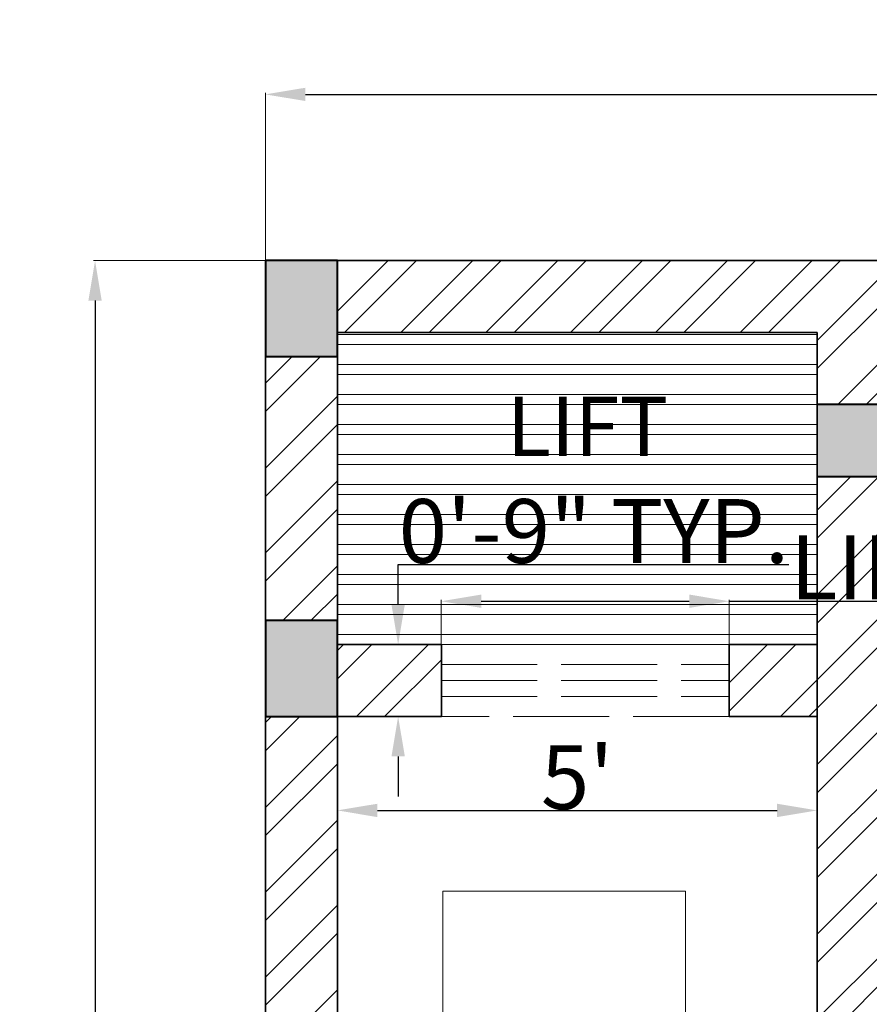
# Model space of a CAD drawing. Units: inches. Extents: x 351 to 1738, y -265 to 286.
# Tile 26 of 38: x 1004 to 1110, y 163 to 286. Entities that reach past the tile are written whole.
import ezdxf

# ---------------------------------------------------------------- set-up
doc = ezdxf.new("R2010")
doc.units = ezdxf.units.IN
doc.header["$MEASUREMENT"] = 0
doc.linetypes.add('ACAD_ISO02W100', pattern=[15, 12, -3])
for name, color, linetype, lineweight in [('A-ANNO-DIMS', 2, 'Continuous', 18), ('A-ANNO-SYMB', 7, 'Continuous', 18), ('A-AREA-IDEN', 7, 'Continuous', 18), ('A-COLS', 7, 'Continuous', 40), ('A-COLS-PATT', 6, 'Continuous', 13), ('A-FLOR-EVTR', 242, 'ACAD_ISO02W100', 18), ('A-FLOR-EVTR-PATT', 9, 'Continuous', 9), ('A-WALL', 7, 'Continuous', 35), ('A-WALL-PATT', 152, 'Continuous', 13)]:
    doc.layers.add(name, color=color, linetype=linetype, lineweight=lineweight)
doc.styles.add('Annotative', font='arial.ttf')
doc.styles.get("Standard").update_dxf_attribs({"font": 'arial.ttf'})
doc.dimstyles.get("Standard").update_dxf_attribs({"dimtxt": 8, "dimasz": 5, "dimexe": 0.18, "dimexo": 0.0625, "dimgap": 0.09, "dimtad": 1, "dimtoh": 1, "dimzin": 0, "dimdsep": 46, "dimlunit": 4, "dimtxsty": 'Standard', "dimcen": 0, "dimclre": 256, "dimadec": 0, "dimazin": 0, "dimtfac": 1, "dimtofl": 0, "dimtmove": 0, "dimatfit": 3, "dimfxl": 1, "dimtolj": 1, "dimtzin": 0, "dimlwe": -1, "dimarcsym": 0})

# ---------------------------------------------------------------- blocks, each defined once
blk = doc.blocks.new('*D7')
at = {"layer": 'A-ANNO-DIMS', "color": 0, "transparency": 16777216}
for p, q in [((1034.7, 256.03), (1034.7, 276.92)), ((1566.7, 256.03), (1566.7, 276.92))]:
    blk.add_line(p, q, dxfattribs=at)
at = {"layer": 'A-ANNO-DIMS', "color": 0, "lineweight": -2, "transparency": 16777216}
blk.add_line((1039.7, 276.74), (1561.7, 276.74), dxfattribs=at)
at = {"layer": 'A-ANNO-DIMS', "color": 0, "transparency": 16777216}
for points in [[(1039.7, 277.57), (1039.7, 275.91), (1034.7, 276.74)], [(1561.7, 277.57), (1561.7, 275.91), (1566.7, 276.74)]]:
    blk.add_solid(points, dxfattribs=at)
at = {"layer": 'Defpoints', "color": 0, "transparency": 16777216}
for p in [(1566.7, 276.74), (1034.7, 255.96), (1566.7, 255.96)]:
    blk.add_point(p, dxfattribs=at)
at = {"layer": 'A-ANNO-DIMS', "color": 0, "transparency": 16777216, "insert": (1300.7, 280.83), "char_height": 8, "attachment_point": 5}
blk.add_mtext('\\A1;44\'-4"', dxfattribs=at)
blk = doc.blocks.new('*D8')
at = {"layer": 'A-ANNO-DIMS', "color": 0, "transparency": 16777216}
for p, q in [((1034.64, 255.96), (1013.22, 255.96)), ((1034.64, -203.04), (1013.22, -203.04))]:
    blk.add_line(p, q, dxfattribs=at)
at = {"layer": 'A-ANNO-DIMS', "color": 0, "lineweight": -2, "transparency": 16777216}
blk.add_line((1013.4, 250.96), (1013.4, -198.04), dxfattribs=at)
at = {"layer": 'A-ANNO-DIMS', "color": 0, "transparency": 16777216}
for points in [[(1012.57, 250.96), (1014.23, 250.96), (1013.4, 255.96)], [(1012.57, -198.04), (1014.23, -198.04), (1013.4, -203.04)]]:
    blk.add_solid(points, dxfattribs=at)
at = {"layer": 'Defpoints', "color": 0, "transparency": 16777216}
for p in [(1034.7, 255.96), (1013.4, -203.04), (1034.7, -203.04)]:
    blk.add_point(p, dxfattribs=at)
at = {"layer": 'A-ANNO-DIMS', "color": 0, "transparency": 16777216, "insert": (1009.22, 26.46), "char_height": 8, "attachment_point": 5, "rotation": 90}
blk.add_mtext('\\A1;38\'-3"', dxfattribs=at)
blk = doc.blocks.new('*D11')
at = {"layer": 'A-ANNO-DIMS', "color": 0, "transparency": 16777216}
for p, q in [((1043.7, 198.9), (1043.7, 187.03)), ((1103.7, 198.9), (1103.7, 187.03))]:
    blk.add_line(p, q, dxfattribs=at)
at = {"layer": 'A-ANNO-DIMS', "color": 0, "lineweight": -2, "transparency": 16777216}
blk.add_line((1048.7, 187.21), (1098.7, 187.21), dxfattribs=at)
at = {"layer": 'A-ANNO-DIMS', "color": 0, "transparency": 16777216}
for points in [[(1048.7, 188.04), (1048.7, 186.37), (1043.7, 187.21)], [(1098.7, 188.04), (1098.7, 186.37), (1103.7, 187.21)]]:
    blk.add_solid(points, dxfattribs=at)
at = {"layer": 'Defpoints', "color": 0, "transparency": 16777216}
for p in [(1043.7, 198.96), (1103.7, 198.96), (1103.7, 187.21)]:
    blk.add_point(p, dxfattribs=at)
at = {"layer": 'A-ANNO-DIMS', "color": 0, "transparency": 16777216, "insert": (1073.7, 191.36), "char_height": 8, "attachment_point": 5}
blk.add_mtext("\\A1;5'", dxfattribs=at)
blk = doc.blocks.new('COL-9x12')
blk.add_lwpolyline([(0, 12), (0, 0), (9, 0), (9, 12)], close=True)
blk = doc.blocks.new('LIFT-DOOR-36')
for p, q in [((0, 9), (36, 9)), ((0, 6.5), (36, 6.5)), ((0, 4.5), (36, 4.5)), ((0, 2.5), (36, 2.5)), ((36, 0), (0, 0))]:
    blk.add_line(p, q)
blk = doc.blocks.new('*D54')
at = {"layer": 'A-ANNO-DIMS', "transparency": 16777216}
for p, q in [((1056.7, 208.03), (1056.7, 213.54)), ((1092.7, 208.03), (1092.7, 213.54))]:
    blk.add_line(p, q, dxfattribs=at)
at = {"layer": 'A-ANNO-DIMS', "color": 0, "lineweight": -2, "transparency": 16777216}
for p, q in [((1061.7, 213.36), (1087.7, 213.36)), ((1092.7, 213.36), (1209.01, 213.36))]:
    blk.add_line(p, q, dxfattribs=at)
at = {"layer": 'A-ANNO-DIMS', "color": 0, "transparency": 16777216}
for points in [[(1061.7, 214.2), (1061.7, 212.53), (1056.7, 213.36)], [(1087.7, 214.2), (1087.7, 212.53), (1092.7, 213.36)]]:
    blk.add_solid(points, dxfattribs=at)
at = {"layer": 'Defpoints', "color": 0, "transparency": 16777216}
for p in [(1092.7, 213.36), (1056.7, 207.96), (1092.7, 207.96)]:
    blk.add_point(p, dxfattribs=at)
at = {"layer": 'A-ANNO-DIMS', "color": 0, "transparency": 16777216, "insert": (1153.35, 217.59), "char_height": 8, "attachment_point": 5}
blk.add_mtext('\\A1;LIFT DOOR 3\'-0" TYP.', dxfattribs=at)
blk = doc.blocks.new('*D55')
at = {"layer": 'A-ANNO-DIMS', "color": 0, "lineweight": -2, "transparency": 16777216}
for p, q in [((1051.3, 212.96), (1051.3, 217.96)), ((1051.3, 217.96), (1100.16, 217.96)), ((1051.3, 193.96), (1051.3, 188.96))]:
    blk.add_line(p, q, dxfattribs=at)
at = {"layer": 'A-ANNO-DIMS', "transparency": 16777216}
for p, q in [((1056.64, 207.96), (1051.12, 207.96)), ((1056.64, 198.96), (1051.12, 198.96))]:
    blk.add_line(p, q, dxfattribs=at)
at = {"layer": 'A-ANNO-DIMS', "color": 0, "transparency": 16777216}
for points in [[(1050.47, 212.96), (1052.14, 212.96), (1051.3, 207.96)], [(1050.47, 193.96), (1052.14, 193.96), (1051.3, 198.96)]]:
    blk.add_solid(points, dxfattribs=at)
at = {"layer": 'Defpoints', "color": 0, "transparency": 16777216}
for p in [(1051.3, 207.96), (1056.7, 207.96), (1056.7, 198.96)]:
    blk.add_point(p, dxfattribs=at)
at = {"layer": 'A-ANNO-DIMS', "color": 0, "transparency": 16777216, "insert": (1075.78, 222.14), "char_height": 8, "attachment_point": 5}
blk.add_mtext('\\A1;0\'-9" TYP.', dxfattribs=at)

msp = doc.modelspace()

# ---------------------------------------------------------------- hatches: boundary and pattern name
at = {"layer": 'A-COLS-PATT'}
h = msp.add_hatch(color=256, dxfattribs=at)
h.dxf.hatch_style = 1
h.paths.add_polyline_path([(1112.704, 237.963), (1103.704, 237.963), (1103.704, 228.963), (1112.704, 228.963)])
h.paths.add_polyline_path([(1115.704, 237.963), (1112.704, 237.963), (1112.704, 228.963), (1115.704, 228.963)])
h.paths.add_polyline_path([(1043.704, 255.963), (1034.704, 255.963), (1034.704, 243.963), (1043.704, 243.963)])
h.paths.add_polyline_path([(1043.704, 210.963), (1034.704, 210.963), (1034.704, 198.963), (1043.704, 198.963)])
h.paths.add_polyline_path([(1043.704, -45.037), (1034.704, -45.037), (1034.704, -57.037), (1043.704, -57.037)])
h.paths.add_polyline_path([(1112.704, -45.037), (1103.704, -45.037), (1103.704, -57.037), (1112.704, -57.037)])
h.paths.add_polyline_path([(1112.704, -161.037), (1103.704, -161.037), (1103.704, -164.037), (1103.704, -173.037), (1112.704, -173.037)])
h.paths.add_polyline_path([(1043.704, -161.037), (1034.704, -161.037), (1034.704, -173.037), (1043.704, -173.037)])
h.paths.add_polyline_path([(1248.549, -164.037), (1236.549, -164.037), (1236.549, -173.037), (1248.549, -173.037)])
h.paths.add_polyline_path([(1248.549, -50), (1236.549, -50), (1236.549, -59), (1248.549, -59)])
h.paths.add_polyline_path([(1248.704, 73.463), (1244.704, 73.463), (1244.704, 64.463), (1248.704, 64.463)])
h.paths.add_polyline_path([(1244.704, 73.463), (1236.704, 73.463), (1236.704, 64.463), (1244.704, 64.463)])
h.paths.add_polyline_path([(1248.704, 237.963), (1236.704, 237.963), (1236.704, 228.963), (1248.704, 228.963)])
h.paths.add_polyline_path([(1392.204, 237.963), (1380.204, 237.963), (1380.204, 228.963), (1392.204, 228.963)])
h.paths.add_polyline_path([(1536.064, 237.963), (1524.064, 237.963), (1524.064, 228.963), (1536.064, 228.963)])
h.paths.add_polyline_path([(1536.064, 73.463), (1524.064, 73.463), (1524.064, 64.463), (1536.064, 64.463)])
h.paths.add_polyline_path([(1384.204, 73.463), (1380.204, 73.463), (1380.204, 64.463), (1384.204, 64.463)])
h.paths.add_polyline_path([(1392.064, 73.463), (1384.204, 73.463), (1384.204, 64.463), (1392.064, 64.463)])
h.paths.add_polyline_path([(1536.064, -53.037), (1524.064, -53.037), (1524.064, -57.037), (1536.064, -57.037)])
h.paths.add_polyline_path([(1536.064, -48.037), (1524.064, -48.037), (1524.064, -53.037), (1536.064, -53.037)])
h.paths.add_polyline_path([(1392.064, -48.037), (1380.064, -48.037), (1380.064, -56.5), (1380.065, -57.037), (1392.064, -57.037)])
h.paths.add_polyline_path([(1536.064, -164.037), (1524.064, -164.037), (1524.064, -173.037), (1536.064, -173.037)])
at = {"layer": 'A-FLOR-EVTR-PATT', "transparency": 33554559}
h = msp.add_hatch(dxfattribs=at)
h.set_pattern_fill('ANSI32', color=256, scale=10, angle=135)
h.set_pattern_definition([(180, (1043.704, 207.9627), (-2e-16, -3.75), []), (180, (1042.454, 209.2127), (-2e-16, -3.75), [])])
h.paths.add_polyline_path([(1103.704, 246.963), (1043.704, 246.963), (1043.704, 243.963), (1043.704, 207.963), (1056.704, 207.963), (1092.704, 207.963), (1103.704, 207.963)])
at = {"layer": 'A-WALL-PATT'}
h = msp.add_hatch(dxfattribs=at)
h.set_pattern_fill('ANSI32', color=256, scale=20)
h.set_pattern_definition([(45, (1034.704, -173.037), (-5.3033, 5.3033), []), (45, (1038.24, -173.037), (-5.3033, 5.3033), [])])
h.paths.add_polyline_path([(1043.704, -57.037), (1034.704, -57.037), (1034.704, -81.037), (1043.704, -81.037)])
h.paths.add_polyline_path([(1043.704, 198.963), (1034.704, 198.963), (1034.704, -45.037), (1043.704, -45.037)])
h.paths.add_polyline_path([(1043.704, 243.963), (1034.704, 243.963), (1034.704, 237.963), (1034.704, 210.963), (1043.704, 210.963)])
h.paths.add_polyline_path([(1112.704, 255.963), (1043.704, 255.963), (1043.704, 246.963), (1103.704, 246.963), (1103.704, 237.963), (1112.704, 237.963), (1112.704, 251.963)])
h.paths.add_polyline_path([(1056.704, 207.963), (1043.704, 207.963), (1043.704, 198.963), (1056.704, 198.963)])
h.paths.add_polyline_path([(1103.704, 207.963), (1092.704, 207.963), (1092.704, 198.963), (1103.704, 198.963)])
h.paths.add_polyline_path([(1112.704, 228.963), (1103.704, 228.963), (1103.704, 74.963), (1112.704, 74.963), (1112.704, 97.5)])
h.paths.add_polyline_path([(1284.129, -164.037), (1248.549, -164.037), (1248.549, -173.037), (1284.129, -173.037)])
h.paths.add_polyline_path([(1524.064, -164.037), (1472.204, -164.037), (1472.204, -138.5), (1468.204, -138.5), (1468.204, -164.037), (1344.129, -164.037), (1344.129, -173.037), (1524.064, -173.037)])
h.paths.add_polyline_path([(1384.204, -57.037), (1380.065, -57.037), (1380.204, -164.037), (1384.204, -164.037)])
h.paths.add_polyline_path([(1566.704, -138), (1557.704, -138), (1557.704, -164.037), (1536.064, -164.037), (1536.064, -173.037), (1566.704, -173.037)])
h.paths.add_polyline_path([(1566.704, -30.189), (1557.704, -30.189), (1557.704, -53.037), (1536.064, -53.037), (1536.064, -57.037), (1557.704, -57.037), (1557.704, -102), (1566.704, -102)])
h.paths.add_polyline_path([(1524.064, -53.037), (1442.549, -53.037), (1442.549, -57.037), (1468.204, -57.037), (1468.204, -102.5), (1472.204, -102.5), (1472.204, -57.037), (1524.064, -57.037)])
h.paths.add_polyline_path([(1566.704, 120.993), (1557.704, 120.993), (1557.704, 29.811), (1566.704, 29.811)])
h.paths.add_polyline_path([(1384.204, 64.463), (1380.204, 64.463), (1380.204, -3.5), (1384.204, -3.5)])
h.paths.add_polyline_path([(1266.549, 237.963), (1248.704, 237.963), (1248.704, 228.963), (1266.549, 228.963)])
h.paths.add_polyline_path([(1329.549, 237.963), (1302.549, 237.963), (1302.549, 228.963), (1329.549, 228.963)])
h.paths.add_polyline_path([(1380.204, 237.963), (1365.549, 237.963), (1365.549, 228.963), (1380.204, 228.963)])
h.paths.add_polyline_path([(1524.064, 237.963), (1392.204, 237.963), (1392.204, 228.963), (1524.064, 228.963)])
h.paths.add_polyline_path([(1384.204, 228.963), (1380.204, 228.963), (1380.204, 73.463), (1384.204, 73.463)])
h.paths.add_polyline_path([(1566.704, 237.963), (1536.064, 237.963), (1536.064, 228.963), (1557.704, 228.963), (1557.704, 180.993), (1566.704, 180.993)])

# ---------------------------------------------------------------- linework, layer by layer
at = {"layer": 'A-ANNO-SYMB'}
msp.add_lwpolyline([(1056.902, -16.259), (1056.902, 177.128), (1087.233, 177.128), (1087.233, 130.616)], dxfattribs=at)
at = {"layer": 'A-COLS'}
msp.add_lwpolyline([(1103.704, 228.963), (1115.704, 228.963), (1115.704, 237.963), (1103.704, 237.963)], dxfattribs=at)
at = {"layer": 'A-WALL'}
for p, q in [((1034.704, 255.963), (1034.704, -81.037)), ((1112.704, 255.963), (1034.704, 255.963)), ((1043.704, 255.963), (1043.704, 207.963)), ((1103.704, 246.963), (1043.704, 246.963)), ((1103.704, 246.963), (1103.704, -57.037)), ((1056.704, 207.963), (1043.704, 207.963)), ((1056.704, 198.963), (1056.704, 207.963)), ((1103.704, 207.963), (1092.704, 207.963)), ((1092.704, 207.963), (1092.704, 198.963)), ((1043.704, 198.963), (1043.704, -81.037)), ((1056.704, 198.963), (1043.704, 198.963)), ((1103.704, 198.963), (1092.704, 198.963))]:
    msp.add_line(p, q, dxfattribs=at)

# ---------------------------------------------------------------- block references
at = {"layer": 'A-COLS'}
for p in [(1034.704, 243.963), (1034.704, 198.963)]:
    msp.add_blockref('COL-9x12', p, dxfattribs=at)
at = {"layer": 'A-FLOR-EVTR'}
msp.add_blockref('LIFT-DOOR-36', (1056.704, 198.963), dxfattribs=at)

# ---------------------------------------------------------------- texts
at = {"layer": 'A-AREA-IDEN', "style": 'Annotative'}
msp.add_text('LIFT', height=7.4326, dxfattribs=at).set_placement((1064.907, 231.521))

# ---------------------------------------------------------------- dimensions: what is measured, and where the dimension line sits
at = {"layer": 'A-ANNO-DIMS'}
dim = msp.add_linear_dim(base=(1566.704, 276.74), p1=(1034.704, 255.963), p2=(1566.704, 255.963), dimstyle='Standard', override={"dimclrd": 0, "dimclre": 0, "dimclrt": 0}, dxfattribs=at)
dim.commit()
dim.dimension.update_dxf_attribs({"geometry": '*D7', "text_midpoint": (1300.704, 280.83)})
dim = msp.add_linear_dim(base=(1013.401, -203.037), p1=(1034.704, 255.963), p2=(1034.704, -203.037), angle=90, dimstyle='Standard', override={"dimclrd": 0, "dimclre": 0, "dimclrt": 0}, dxfattribs=at)
dim.commit()
dim.dimension.update_dxf_attribs({"geometry": '*D8', "text_midpoint": (1013.401, 26.463), "dimtype": 160})
dim = msp.add_linear_dim(base=(1092.704, 213.363), p1=(1056.704, 207.963), p2=(1092.704, 207.963), text='LIFT DOOR <> TYP.', dimstyle='Standard', override={"dimdec": 1, "dimlfac": 1, "dimrnd": 0, "dimzin": 1, "dimdsep": 46, "dimlunit": 4, "dimfrac": 2}, dxfattribs=at)
dim.commit()
dim.dimension.update_dxf_attribs({"geometry": '*D54', "text_midpoint": (1153.355, 217.595)})
dim = msp.add_linear_dim(base=(1051.304, 207.963), p1=(1056.704, 198.963), p2=(1056.704, 207.963), angle=90, text='<> TYP.', dimstyle='Standard', override={"dimdec": 1, "dimlfac": 1, "dimrnd": 0, "dimzin": 1, "dimdsep": 46, "dimlunit": 4, "dimfrac": 2}, dxfattribs=at)
dim.commit()
dim.dimension.update_dxf_attribs({"geometry": '*D55', "text_midpoint": (1075.776, 222.137)})
dim = msp.add_linear_dim(base=(1103.704, 187.205), p1=(1043.704, 198.963), p2=(1103.704, 198.963), dimstyle='Standard', override={"dimclrd": 0, "dimclre": 0, "dimclrt": 0}, dxfattribs=at)
dim.commit()
dim.dimension.update_dxf_attribs({"geometry": '*D11', "text_midpoint": (1073.704, 187.205), "dimtype": 160})

doc.saveas('drawing.dxf')
